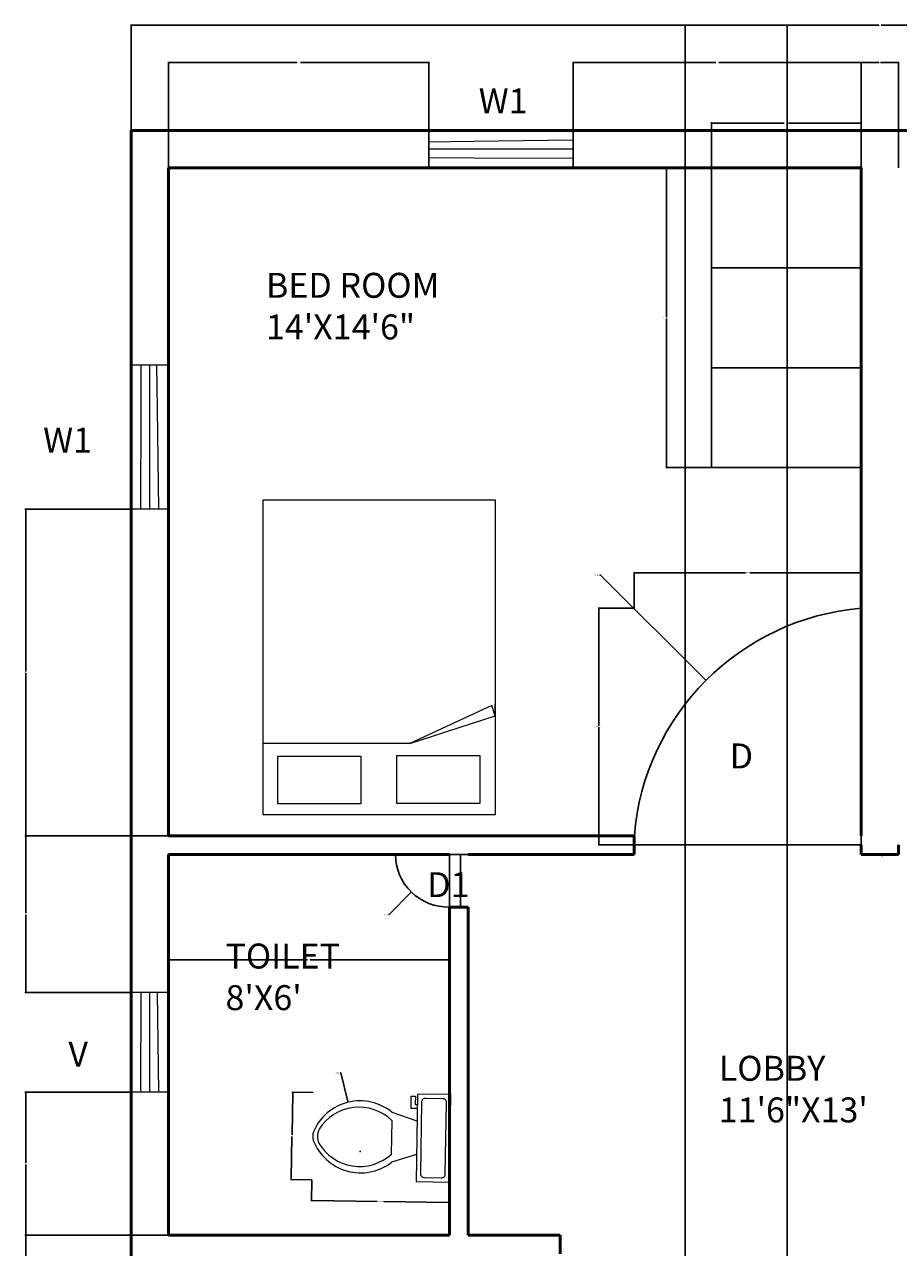
# Model space of a CAD drawing. Units: inches. Extents: x 2521 to 2933, y 1745 to 2276.
# Tile 3 of 4: x 2521 to 2731, y 1982 to 2276. Entities that reach past the tile are written whole.
import ezdxf

# ---------------------------------------------------------------- set-up
doc = ezdxf.new("R2010")
doc.units = ezdxf.units.IN
for name, color, linetype, lineweight in [('A-ANNO-DIMS', 2, 'Continuous', 18), ('A-ANNO-TEXT', 3, 'Continuous', 18), ('A-AREA-IDEN', 7, 'Continuous', 25), ('A-DOOR', 3, 'Continuous', 25), ('A-FLOR-CASE', 32, 'Continuous', 25), ('A-FLOR-FIXT', 9, 'Continuous', 18), ('A-FURN', 8, 'Continuous', 18), ('A-GLAZ', 4, 'Continuous', 20), ('A-WALL', 7, 'Continuous', 50)]:
    doc.layers.add(name, color=color, linetype=linetype, lineweight=lineweight)
doc.styles.get("Standard").update_dxf_attribs({"font": 'arial.ttf'})
doc.dimstyles.get("Standard").update_dxf_attribs({"dimtxt": 0.18, "dimasz": 0.18, "dimexe": 0.18, "dimexo": 0.0625, "dimgap": 0.09, "dimtad": 0, "dimtih": 1, "dimtoh": 1, "dimdec": 4, "dimzin": 0, "dimdsep": 46, "dimtxsty": 'Standard', "dimcen": 0.09, "dimadec": 0, "dimazin": 0, "dimtfac": 1, "dimtdec": 4, "dimtofl": 0, "dimtmove": 0, "dimatfit": 3, "dimfxl": 1, "dimtolj": 1, "dimtzin": 0, "dimarcsym": 0})

# ---------------------------------------------------------------- blocks, each defined once
blk = doc.blocks.new('Toilet - top')
for p, q in [((9.5, -6), (9.5, -2)), ((-10, -8.5), (-8, -8.5)), ((-10, -9.5), (-10, -8.5)), ((-8, -8.5), (-8, -8)), ((-7, -8), (-7, -9.5)), ((-4, -8), (-6, -14)), ((4, -8), (6, -14)), ((-7, -9.5), (-10, -9.5)), ((4, -14), (-4, -14))]:
    blk.add_line(p, q)
blk.add_lwpolyline([(10.5, -8), (10.5, 0), (-10.5, 0), (-10.5, -8)], close=True)
for points in [[(-9.5, -2), (-9.5, -6)], [(8.5, -1), (-8.5, -1)], [(-8.5, -7), (8.5, -7)]]:
    blk.add_lwpolyline(points)
for centre, radius, start, end in [((-8.62, -1.88), 0.884, 81.8699, 188.1301), ((8.62, -1.88), 0.884, 351.8699, 98.1301), ((-8.62, -6.12), 0.884, 171.8699, 278.1301), ((8.62, -6.12), 0.884, 261.8699, 8.1301), ((3.52, -21.58), 12.17, 141.4691, 247.9714), ((4.2, -21.82), 11.33, 136.3677, 238.9468), ((-3.52, -21.58), 12.17, 292.0284, 38.5307), ((-4.2, -21.82), 11.33, 301.053, 43.6321), ((0, -27.88), 4, 245.7318, 294.2682), ((0, -29), 4, 254.8605, 285.1395)]:
    blk.add_arc(centre, radius, start, end)
blk = doc.blocks.new('WINDOW-W1-LONG')
for p, q in [((0, 24), (0, 34.69)), ((0, 34.69), (9, 34.69)), ((2.4, 24), (2.44, 34.69)), ((4.5, 24), (4.5, 34.69)), ((6.37, 24), (6.23, 34.69)), ((9, 34.69), (9, 24)), ((0, 24), (0, 0)), ((2.32, 0), (2.4, 24)), ((4.5, 0), (4.5, 24)), ((6.68, 0), (6.37, 24)), ((9, 24), (9, 0)), ((9, 0), (0, 0))]:
    blk.add_line(p, q)
blk = doc.blocks.new('WINDOW-24')
for p, q in [((9, 24), (0, 24)), ((0, 24), (0, 0)), ((2.32, 0), (2.4, 24)), ((4.5, 0), (4.5, 24)), ((6.68, 0), (6.37, 24)), ((9, 24), (9, 0)), ((9, 0), (0, 0))]:
    blk.add_line(p, q)
blk = doc.blocks.new('DOOR-SINGLE-SWING')
for p, q in [((54.54, 0), (54.54, 56.86)), ((0, 0), (54.54, 0))]:
    blk.add_line(p, q)
blk.add_arc((59.46, -2.59), 59.65, 94.7338, 175.398)
blk = doc.blocks.new('BED-DOUBLE')
for p, q in [((55.72, 23.76), (55.72, 26.62)), ((54.9, 26.24), (35.19, 17.12)), ((35.19, 17.12), (55.72, 23.76)), ((55.72, 23.76), (54.9, 26.24)), ((35.19, 17.12), (0, 17.12))]:
    blk.add_line(p, q)
for points in [[(0, 75.73), (55.72, 75.73), (55.72, 0), (0, 0)], [(3.53, 14.11), (23.44, 14.11), (23.44, 2.6), (3.53, 2.6)], [(32.11, 14.25), (52.02, 14.25), (52.02, 2.74), (32.11, 2.74)]]:
    blk.add_lwpolyline(points, close=True)
blk = doc.blocks.new('CABINET-3-BAY')
for p, q in [((0, 0), (0, 72)), ((0, 48), (36, 48)), ((0, 24), (36, 24)), ((0, 0), (36, 0))]:
    blk.add_line(p, q)
blk = doc.blocks.new('*D15')
at = {"layer": 'A-ANNO-DIMS', "color": 0, "lineweight": -2, "transparency": 16777216}
for p, q in [((2686.45, 2241.28), (2675.53, 2241.28)), ((2675.71, 2241.1), (2675.71, 2205.46)), ((2675.71, 2169.46), (2675.71, 2205.1)), ((2686.45, 2169.28), (2675.53, 2169.28))]:
    blk.add_line(p, q, dxfattribs=at)
at = {"layer": 'A-ANNO-DIMS', "color": 0, "transparency": 16777216}
for points in [[(2675.68, 2241.1), (2675.74, 2241.1), (2675.71, 2241.28)], [(2675.68, 2169.46), (2675.74, 2169.46), (2675.71, 2169.28)]]:
    blk.add_solid(points, dxfattribs=at)
at = {"layer": 'Defpoints', "color": 0, "transparency": 16777216}
for p in [(2675.71, 2241.28), (2686.51, 2241.28), (2686.51, 2169.28)]:
    blk.add_point(p, dxfattribs=at)
at = {"layer": 'A-ANNO-DIMS', "color": 0, "transparency": 16777216, "insert": (2675.71, 2205.28), "char_height": 0.18, "attachment_point": 5}
blk.add_mtext('\\A1;CABINET 72 TYP.', dxfattribs=at)
blk = doc.blocks.new('*D16')
at = {"layer": 'A-ANNO-DIMS', "color": 0, "lineweight": -2, "transparency": 16777216}
for p, q in [((2686.51, 2241.34), (2686.51, 2252.26)), ((2686.69, 2252.08), (2703.98, 2252.08)), ((2722.33, 2252.08), (2705.04, 2252.08)), ((2722.51, 2241.34), (2722.51, 2252.26))]:
    blk.add_line(p, q, dxfattribs=at)
at = {"layer": 'A-ANNO-DIMS', "color": 0, "transparency": 16777216}
for points in [[(2686.69, 2252.11), (2686.69, 2252.05), (2686.51, 2252.08)], [(2722.33, 2252.11), (2722.33, 2252.05), (2722.51, 2252.08)]]:
    blk.add_solid(points, dxfattribs=at)
at = {"layer": 'Defpoints', "color": 0, "transparency": 16777216}
for p in [(2722.51, 2252.08), (2686.51, 2241.28), (2722.51, 2241.28)]:
    blk.add_point(p, dxfattribs=at)
at = {"layer": 'A-ANNO-DIMS', "color": 0, "transparency": 16777216, "insert": (2704.51, 2252.08), "char_height": 0.18, "attachment_point": 5}
blk.add_mtext('\\A1;36 TYP.', dxfattribs=at)
blk = doc.blocks.new('*D17')
at = {"layer": 'A-ANNO-DIMS', "color": 0, "lineweight": -2, "transparency": 16777216}
for p, q in [((2667.91, 2135.44), (2659.26, 2135.44)), ((2659.44, 2135.26), (2659.44, 2107.2)), ((2659.44, 2078.77), (2659.44, 2106.83)), ((2667.91, 2078.59), (2659.26, 2078.59))]:
    blk.add_line(p, q, dxfattribs=at)
at = {"layer": 'A-ANNO-DIMS', "color": 0, "transparency": 16777216}
for points in [[(2659.41, 2135.26), (2659.47, 2135.26), (2659.44, 2135.44)], [(2659.41, 2078.77), (2659.47, 2078.77), (2659.44, 2078.59)]]:
    blk.add_solid(points, dxfattribs=at)
at = {"layer": 'Defpoints', "color": 0, "transparency": 16777216}
for p in [(2659.44, 2135.44), (2667.97, 2135.44), (2667.97, 2078.59)]:
    blk.add_point(p, dxfattribs=at)
at = {"layer": 'A-ANNO-DIMS', "color": 0, "transparency": 16777216, "insert": (2659.44, 2107.01), "char_height": 0.18, "attachment_point": 5}
blk.add_mtext('\\A1;DOOR 57 TYP.', dxfattribs=at)
blk = doc.blocks.new('*D18')
at = {"layer": 'A-ANNO-DIMS', "color": 0, "lineweight": -2, "transparency": 16777216}
for p, q in [((2667.97, 2135.51), (2667.97, 2144.15)), ((2668.15, 2143.97), (2694.71, 2143.97)), ((2722.33, 2143.97), (2695.77, 2143.97)), ((2722.51, 2135.51), (2722.51, 2144.15))]:
    blk.add_line(p, q, dxfattribs=at)
at = {"layer": 'A-ANNO-DIMS', "color": 0, "transparency": 16777216}
for points in [[(2668.15, 2144), (2668.15, 2143.94), (2667.97, 2143.97)], [(2722.33, 2144), (2722.33, 2143.94), (2722.51, 2143.97)]]:
    blk.add_solid(points, dxfattribs=at)
at = {"layer": 'Defpoints', "color": 0, "transparency": 16777216}
for p in [(2722.51, 2143.97), (2667.97, 2135.44), (2722.51, 2135.44)]:
    blk.add_point(p, dxfattribs=at)
at = {"layer": 'A-ANNO-DIMS', "color": 0, "transparency": 16777216, "insert": (2695.24, 2143.97), "char_height": 0.18, "attachment_point": 5}
blk.add_mtext('\\A1;55 TYP.', dxfattribs=at)
blk = doc.blocks.new('*D19')
at = {"layer": 'A-ANNO-DIMS', "color": 0, "lineweight": -2, "transparency": 16777216}
for p, q in [((2590.47, 1998.02), (2590.38, 1992.94)), ((2623.51, 1997.47), (2623.42, 1992.4)), ((2590.57, 1993.12), (2606.13, 1992.86)), ((2623.25, 1992.58), (2607.68, 1992.84))]:
    blk.add_line(p, q, dxfattribs=at)
at = {"layer": 'A-ANNO-DIMS', "color": 0, "transparency": 16777216}
for points in [[(2590.57, 1993.15), (2590.57, 1993.09), (2590.39, 1993.12)], [(2623.25, 1992.61), (2623.25, 1992.55), (2623.43, 1992.58)]]:
    blk.add_solid(points, dxfattribs=at)
at = {"layer": 'Defpoints', "color": 0, "transparency": 16777216}
for p in [(2590.47, 1998.08), (2623.51, 1997.53), (2623.43, 1992.58)]:
    blk.add_point(p, dxfattribs=at)
at = {"layer": 'A-ANNO-DIMS', "color": 0, "transparency": 16777216, "insert": (2606.91, 1992.85), "char_height": 0.18, "attachment_point": 5}
blk.add_mtext('\\A1;WC 33 TYP.', dxfattribs=at)
blk = doc.blocks.new('*D20')
at = {"layer": 'A-ANNO-DIMS', "color": 0, "lineweight": -2, "transparency": 16777216}
for p, q in [((2590.75, 2019.08), (2585.68, 2019.16)), ((2585.85, 2018.98), (2585.69, 2008.84)), ((2585.51, 1998.34), (2585.68, 2008.48)), ((2590.4, 1998.08), (2585.33, 1998.16))]:
    blk.add_line(p, q, dxfattribs=at)
at = {"layer": 'A-ANNO-DIMS', "color": 0, "transparency": 16777216}
for points in [[(2585.82, 2018.98), (2585.88, 2018.98), (2585.86, 2019.16)], [(2585.48, 1998.34), (2585.54, 1998.34), (2585.51, 1998.16)]]:
    blk.add_solid(points, dxfattribs=at)
at = {"layer": 'Defpoints', "color": 0, "transparency": 16777216}
for p in [(2590.81, 2019.08), (2585.51, 1998.16), (2590.47, 1998.08)]:
    blk.add_point(p, dxfattribs=at)
at = {"layer": 'A-ANNO-DIMS', "color": 0, "transparency": 16777216, "insert": (2585.68, 2008.66), "char_height": 0.18, "attachment_point": 5}
blk.add_mtext('\\A1;21 TYP.', dxfattribs=at)
blk = doc.blocks.new('*D23')
at = {"layer": 'A-ANNO-DIMS', "color": 0, "lineweight": -2, "transparency": 16777216}
for p, q in [((2547.01, 2250.34), (2547.01, 2275.78)), ((2547.19, 2275.6), (2726.72, 2275.6)), ((2906.83, 2275.6), (2727.3, 2275.6)), ((2907.01, 2250.34), (2907.01, 2275.78))]:
    blk.add_line(p, q, dxfattribs=at)
at = {"layer": 'A-ANNO-DIMS', "color": 0, "transparency": 16777216}
for points in [[(2547.19, 2275.63), (2547.19, 2275.57), (2547.01, 2275.6)], [(2906.83, 2275.63), (2906.83, 2275.57), (2907.01, 2275.6)]]:
    blk.add_solid(points, dxfattribs=at)
at = {"layer": 'Defpoints', "color": 0, "transparency": 16777216}
for p in [(2907.01, 2275.6), (2547.01, 2250.28), (2907.01, 2250.28)]:
    blk.add_point(p, dxfattribs=at)
at = {"layer": 'A-ANNO-DIMS', "color": 0, "transparency": 16777216, "insert": (2727.01, 2275.6), "char_height": 0.18, "attachment_point": 5}
blk.add_mtext('\\A1;360', dxfattribs=at)
blk = doc.blocks.new('*D25')
at = {"layer": 'A-ANNO-DIMS', "color": 0, "lineweight": -2, "transparency": 16777216}
for p, q in [((2556.01, 2241.34), (2556.01, 2266.78)), ((2618.6, 2241.34), (2618.6, 2266.78)), ((2556.19, 2266.6), (2586.91, 2266.6)), ((2618.42, 2266.6), (2587.7, 2266.6))]:
    blk.add_line(p, q, dxfattribs=at)
at = {"layer": 'A-ANNO-DIMS', "color": 0, "transparency": 16777216}
for points in [[(2556.19, 2266.63), (2556.19, 2266.57), (2556.01, 2266.6)], [(2618.42, 2266.63), (2618.42, 2266.57), (2618.6, 2266.6)]]:
    blk.add_solid(points, dxfattribs=at)
at = {"layer": 'Defpoints', "color": 0, "transparency": 16777216}
for p in [(2618.6, 2266.6), (2556.01, 2241.28), (2618.6, 2241.28)]:
    blk.add_point(p, dxfattribs=at)
at = {"layer": 'A-ANNO-DIMS', "color": 0, "transparency": 16777216, "insert": (2587.31, 2266.6), "char_height": 0.18, "attachment_point": 5}
blk.add_mtext('\\A1;62.59', dxfattribs=at)
blk = doc.blocks.new('*D26')
at = {"layer": 'A-ANNO-DIMS', "color": 0, "lineweight": -2, "transparency": 16777216}
for p, q in [((2653.3, 2241.34), (2653.3, 2266.78)), ((2722.51, 2241.34), (2722.51, 2266.78)), ((2653.48, 2266.6), (2687.53, 2266.6)), ((2722.33, 2266.6), (2688.28, 2266.6))]:
    blk.add_line(p, q, dxfattribs=at)
at = {"layer": 'A-ANNO-DIMS', "color": 0, "transparency": 16777216}
for points in [[(2653.48, 2266.63), (2653.48, 2266.57), (2653.3, 2266.6)], [(2722.33, 2266.63), (2722.33, 2266.57), (2722.51, 2266.6)]]:
    blk.add_solid(points, dxfattribs=at)
at = {"layer": 'Defpoints', "color": 0, "transparency": 16777216}
for p in [(2722.51, 2266.6), (2653.3, 2241.28), (2722.51, 2241.28)]:
    blk.add_point(p, dxfattribs=at)
at = {"layer": 'A-ANNO-DIMS', "color": 0, "transparency": 16777216, "insert": (2687.9, 2266.6), "char_height": 0.18, "attachment_point": 5}
blk.add_mtext('\\A1;69.21', dxfattribs=at)
blk = doc.blocks.new('*D27')
at = {"layer": 'A-ANNO-DIMS', "color": 0, "lineweight": -2, "transparency": 16777216}
for p, q in [((2722.51, 2241.34), (2722.51, 2266.78)), ((2731.51, 2241.34), (2731.51, 2266.78)), ((2722.69, 2266.6), (2726.86, 2266.6)), ((2731.33, 2266.6), (2727.16, 2266.6))]:
    blk.add_line(p, q, dxfattribs=at)
at = {"layer": 'A-ANNO-DIMS', "color": 0, "transparency": 16777216}
for points in [[(2722.69, 2266.63), (2722.69, 2266.57), (2722.51, 2266.6)], [(2731.33, 2266.63), (2731.33, 2266.57), (2731.51, 2266.6)]]:
    blk.add_solid(points, dxfattribs=at)
at = {"layer": 'Defpoints', "color": 0, "transparency": 16777216}
for p in [(2731.51, 2266.6), (2722.51, 2241.28), (2731.51, 2241.28)]:
    blk.add_point(p, dxfattribs=at)
at = {"layer": 'A-ANNO-DIMS', "color": 0, "transparency": 16777216, "insert": (2727.01, 2266.6), "char_height": 0.18, "attachment_point": 5}
blk.add_mtext('\\A1;9', dxfattribs=at)
blk = doc.blocks.new('*D31')
at = {"layer": 'A-ANNO-DIMS', "color": 0, "lineweight": -2, "transparency": 16777216}
for p, q in [((2555.95, 1984.78), (2521.51, 1984.78)), ((2521.69, 1984.6), (2521.69, 1937.71)), ((2521.69, 1890.46), (2521.69, 1937.35)), ((2555.95, 1890.28), (2521.51, 1890.28))]:
    blk.add_line(p, q, dxfattribs=at)
at = {"layer": 'A-ANNO-DIMS', "color": 0, "transparency": 16777216}
for points in [[(2521.66, 1984.6), (2521.72, 1984.6), (2521.69, 1984.78)], [(2521.66, 1890.46), (2521.72, 1890.46), (2521.69, 1890.28)]]:
    blk.add_solid(points, dxfattribs=at)
at = {"layer": 'Defpoints', "color": 0, "transparency": 16777216}
for p in [(2521.69, 1984.78), (2556.01, 1984.78), (2556.01, 1890.28)]:
    blk.add_point(p, dxfattribs=at)
at = {"layer": 'A-ANNO-DIMS', "color": 0, "transparency": 16777216, "insert": (2521.69, 1937.53), "char_height": 0.18, "attachment_point": 5}
blk.add_mtext('\\A1;94.5', dxfattribs=at)
blk = doc.blocks.new('*D32')
at = {"layer": 'A-ANNO-DIMS', "color": 0, "lineweight": -2, "transparency": 16777216}
for p, q in [((2546.95, 2019.1), (2521.51, 2019.1)), ((2521.69, 2018.92), (2521.69, 2002.12)), ((2521.69, 1984.96), (2521.69, 2001.76)), ((2555.95, 1984.78), (2521.51, 1984.78))]:
    blk.add_line(p, q, dxfattribs=at)
at = {"layer": 'A-ANNO-DIMS', "color": 0, "transparency": 16777216}
for points in [[(2521.66, 2018.92), (2521.72, 2018.92), (2521.69, 2019.1)], [(2521.66, 1984.96), (2521.72, 1984.96), (2521.69, 1984.78)]]:
    blk.add_solid(points, dxfattribs=at)
at = {"layer": 'Defpoints', "color": 0, "transparency": 16777216}
for p in [(2521.69, 2019.1), (2547.01, 2019.1), (2556.01, 1984.78)]:
    blk.add_point(p, dxfattribs=at)
at = {"layer": 'A-ANNO-DIMS', "color": 0, "transparency": 16777216, "insert": (2521.69, 2001.94), "char_height": 0.18, "attachment_point": 5}
blk.add_mtext('\\A1;34.32', dxfattribs=at)
blk = doc.blocks.new('*D33')
at = {"layer": 'A-ANNO-DIMS', "color": 0, "lineweight": -2, "transparency": 16777216}
for p, q in [((2555.95, 2080.78), (2521.51, 2080.78)), ((2521.69, 2080.6), (2521.69, 2062.12)), ((2521.69, 2043.28), (2521.69, 2061.76)), ((2546.95, 2043.1), (2521.51, 2043.1))]:
    blk.add_line(p, q, dxfattribs=at)
at = {"layer": 'A-ANNO-DIMS', "color": 0, "transparency": 16777216}
for points in [[(2521.66, 2080.6), (2521.72, 2080.6), (2521.69, 2080.78)], [(2521.66, 2043.28), (2521.72, 2043.28), (2521.69, 2043.1)]]:
    blk.add_solid(points, dxfattribs=at)
at = {"layer": 'Defpoints', "color": 0, "transparency": 16777216}
for p in [(2521.69, 2080.78), (2556.01, 2080.78), (2547.01, 2043.1)]:
    blk.add_point(p, dxfattribs=at)
at = {"layer": 'A-ANNO-DIMS', "color": 0, "transparency": 16777216, "insert": (2521.69, 2061.94), "char_height": 0.18, "attachment_point": 5}
blk.add_mtext('\\A1;37.68', dxfattribs=at)
blk = doc.blocks.new('*D34')
at = {"layer": 'A-ANNO-DIMS', "color": 0, "lineweight": -2, "transparency": 16777216}
for p, q in [((2546.95, 2159.3), (2521.51, 2159.3)), ((2521.69, 2159.12), (2521.69, 2120.22)), ((2521.69, 2080.96), (2521.69, 2119.86)), ((2555.95, 2080.78), (2521.51, 2080.78))]:
    blk.add_line(p, q, dxfattribs=at)
at = {"layer": 'A-ANNO-DIMS', "color": 0, "transparency": 16777216}
for points in [[(2521.66, 2159.12), (2521.72, 2159.12), (2521.69, 2159.3)], [(2521.66, 2080.96), (2521.72, 2080.96), (2521.69, 2080.78)]]:
    blk.add_solid(points, dxfattribs=at)
at = {"layer": 'Defpoints', "color": 0, "transparency": 16777216}
for p in [(2521.69, 2159.3), (2547.01, 2159.3), (2556.01, 2080.78)]:
    blk.add_point(p, dxfattribs=at)
at = {"layer": 'A-ANNO-DIMS', "color": 0, "transparency": 16777216, "insert": (2521.69, 2120.04), "char_height": 0.18, "attachment_point": 5}
blk.add_mtext('\\A1;78.51', dxfattribs=at)
blk = doc.blocks.new('*D48')
at = {"layer": 'A-ANNO-DIMS', "color": 0, "lineweight": -2, "transparency": 16777216}
for p, q in [((2556.01, 2076.22), (2556.01, 2050.78)), ((2623.51, 2076.22), (2623.51, 2050.78)), ((2556.19, 2050.96), (2589.43, 2050.96)), ((2623.33, 2050.96), (2590.08, 2050.96))]:
    blk.add_line(p, q, dxfattribs=at)
at = {"layer": 'A-ANNO-DIMS', "color": 0, "transparency": 16777216}
for points in [[(2556.19, 2050.99), (2556.19, 2050.93), (2556.01, 2050.96)], [(2623.33, 2050.99), (2623.33, 2050.93), (2623.51, 2050.96)]]:
    blk.add_solid(points, dxfattribs=at)
at = {"layer": 'Defpoints', "color": 0, "transparency": 16777216}
for p in [(2556.01, 2076.28), (2623.51, 2076.28), (2556.01, 2050.96)]:
    blk.add_point(p, dxfattribs=at)
at = {"layer": 'A-ANNO-DIMS', "color": 0, "transparency": 16777216, "insert": (2589.76, 2050.96), "char_height": 0.18, "attachment_point": 5}
blk.add_mtext('\\A1;67.5', dxfattribs=at)
blk = doc.blocks.new('*D55')
at = {"layer": 'A-ANNO-DIMS', "color": 0, "lineweight": -2, "transparency": 16777216}
for p, q in [((2680.23, 1804.66), (2680.23, 2275.78)), ((2680.41, 2275.6), (2692.15, 2275.6)), ((2704.55, 2275.6), (2692.81, 2275.6)), ((2704.73, 1859.95), (2704.73, 2275.78))]:
    blk.add_line(p, q, dxfattribs=at)
at = {"layer": 'A-ANNO-DIMS', "color": 0, "transparency": 16777216}
for points in [[(2680.41, 2275.63), (2680.41, 2275.57), (2680.23, 2275.6)], [(2704.55, 2275.63), (2704.55, 2275.57), (2704.73, 2275.6)]]:
    blk.add_solid(points, dxfattribs=at)
at = {"layer": 'Defpoints', "color": 0, "transparency": 16777216}
for p in [(2704.73, 2275.6), (2704.73, 1859.89), (2680.23, 1804.6)]:
    blk.add_point(p, dxfattribs=at)
at = {"layer": 'A-ANNO-DIMS', "color": 0, "transparency": 16777216, "insert": (2692.48, 2275.6), "char_height": 0.18, "attachment_point": 5}
blk.add_mtext('\\A1;24.5', dxfattribs=at)
blk = doc.blocks.new('*D61')
at = {"layer": 'A-ANNO-DIMS', "color": 0, "lineweight": -2, "transparency": 16777216}
for p, q in [((2659.69, 2143.41), (2659.87, 2143.41)), ((2659.87, 2143.41), (2685.08, 2118.25)), ((2727.34, 2076), (2727.52, 2076)), ((2727.43, 2075.91), (2727.43, 2076.09))]:
    blk.add_line(p, q, dxfattribs=at)
at = {"layer": 'A-ANNO-DIMS', "color": 0, "transparency": 16777216}
blk.add_solid([(2685.1, 2118.28), (2685.06, 2118.23), (2685.2, 2118.13)], dxfattribs=at)
at = {"layer": 'Defpoints', "color": 0, "transparency": 16777216}
for p in [(2685.2, 2118.13), (2727.43, 2076)]:
    blk.add_point(p, dxfattribs=at)
at = {"layer": 'A-ANNO-DIMS', "color": 0, "transparency": 16777216, "insert": (2659.01, 2143.41), "char_height": 0.18, "attachment_point": 5}
blk.add_mtext('\\A1;2X R59.65', dxfattribs=at)
blk = doc.blocks.new('*D63')
at = {"layer": 'A-ANNO-DIMS', "color": 0, "lineweight": -2, "transparency": 16777216}
for p, q in [((2623.12, 2076.24), (2623.3, 2076.24)), ((2623.21, 2076.15), (2623.21, 2076.33)), ((2609.07, 2061.81), (2614.25, 2067.1)), ((2608.89, 2061.81), (2609.07, 2061.81))]:
    blk.add_line(p, q, dxfattribs=at)
at = {"layer": 'A-ANNO-DIMS', "color": 0, "transparency": 16777216}
blk.add_solid([(2614.23, 2067.12), (2614.27, 2067.07), (2614.38, 2067.22)], dxfattribs=at)
at = {"layer": 'Defpoints', "color": 0, "transparency": 16777216}
for p in [(2623.21, 2076.24), (2614.38, 2067.22)]:
    blk.add_point(p, dxfattribs=at)
at = {"layer": 'A-ANNO-DIMS', "color": 0, "transparency": 16777216, "insert": (2608.34, 2061.81), "char_height": 0.18, "attachment_point": 5}
blk.add_mtext('\\A1;R12.627', dxfattribs=at)
blk = doc.blocks.new('*D64')
at = {"layer": 'A-ANNO-DIMS', "color": 0, "lineweight": -2, "transparency": 16777216}
for p, q in [((2597.23, 2023.78), (2597.41, 2023.78)), ((2597.41, 2023.78), (2599.11, 2016.86)), ((2601.96, 2004.87), (2602.14, 2004.87)), ((2602.05, 2004.78), (2602.05, 2004.96))]:
    blk.add_line(p, q, dxfattribs=at)
at = {"layer": 'A-ANNO-DIMS', "color": 0, "transparency": 16777216}
blk.add_solid([(2599.13, 2016.87), (2599.08, 2016.86), (2599.15, 2016.69)], dxfattribs=at)
at = {"layer": 'Defpoints', "color": 0, "transparency": 16777216}
for p in [(2599.15, 2016.69), (2602.05, 2004.87)]:
    blk.add_point(p, dxfattribs=at)
at = {"layer": 'A-ANNO-DIMS', "color": 0, "transparency": 16777216, "insert": (2596.55, 2023.78), "char_height": 0.18, "attachment_point": 5}
blk.add_mtext('\\A1;4X R12.17', dxfattribs=at)

msp = doc.modelspace()

# ---------------------------------------------------------------- linework, layer by layer
at = {"layer": 'A-DOOR'}
for p, q in [((2610.5844, 2076.2819), (2626.1881, 2076.2819)), ((2626.1881, 2076.2819), (2626.1881, 2063.9735)), ((2628.009, 2076.2819), (2626.1881, 2076.2819)), ((2626.1881, 2063.9735), (2626.1881, 2063.6098))]:
    msp.add_line(p, q, dxfattribs=at)
msp.add_arc((2623.2111, 2076.2443), 12.6267, 179.82927, 271.352003, dxfattribs=at)
at = {"layer": 'A-WALL'}
for p, q in [((2547.009, 2250.2819), (2907.009, 2250.2819)), ((2547.009, 1770.2819), (2547.009, 2250.2819)), ((2556.009, 2241.2819), (2722.509, 2241.2819)), ((2556.009, 2080.7819), (2556.009, 2241.2819)), ((2722.509, 2080.7819), (2722.509, 2241.2819)), ((2667.9735, 2080.7819), (2556.009, 2080.7819)), ((2667.9735, 2080.7819), (2667.9735, 2076.2819)), ((2722.509, 2078.585), (2722.509, 2076.2819)), ((2731.479, 2078.585), (2731.479, 2076.2819)), ((2556.009, 2076.2819), (2556.009, 1984.7819)), ((2556.009, 1984.7819), (2556.009, 2076.2819)), ((2623.509, 2076.2819), (2556.009, 2076.2819)), ((2667.9735, 2076.2819), (2628.009, 2076.2819)), ((2722.509, 2076.2819), (2731.479, 2076.2819)), ((2623.509, 1984.7819), (2623.509, 2063.621)), ((2623.509, 2063.621), (2628.009, 2063.6022)), ((2628.009, 1984.7819), (2628.009, 2063.6022)), ((2556.009, 1984.7819), (2623.509, 1984.7819)), ((2628.009, 1984.7819), (2650.1821, 1984.7819)), ((2650.1821, 1980.2819), (2650.1821, 1984.7819))]:
    msp.add_line(p, q, dxfattribs=at)

# ---------------------------------------------------------------- block references
at = {"layer": 'A-DOOR'}
msp.add_blockref('DOOR-SINGLE-SWING', (2667.973, 2078.585), dxfattribs=at)
at = {"layer": 'A-FLOR-CASE'}
msp.add_blockref('CABINET-3-BAY', (2686.509, 2169.282), dxfattribs=at)
at = {"layer": 'A-FLOR-FIXT', "rotation": 269.0579063208954}
msp.add_blockref('Toilet - top', (2623.6817, 2008.0334), dxfattribs=at)
at = {"layer": 'A-FURN'}
msp.add_blockref('BED-DOUBLE', (2578.788, 2085.81), dxfattribs=at)
at = {"layer": 'A-GLAZ', "rotation": 89.99999999999793}
msp.add_blockref('WINDOW-W1-LONG', (2653.2972, 2241.2819), dxfattribs=at)
at = {"layer": 'A-GLAZ'}
for name, p in [('WINDOW-W1-LONG', (2547.009, 2159.295)), ('WINDOW-24', (2547.009, 2019.1009))]:
    msp.add_blockref(name, p, dxfattribs=at)

# ---------------------------------------------------------------- texts
at = {"layer": 'A-ANNO-TEXT', "char_height": 6, "attachment_point": 1}
for s, width, insert in [('W1', 10.7254, (2630.5716, 2260.4013)), ('W1', 15.32248, (2525.8777, 2178.8496)), ('D', 9.612648, (2690.8877, 2102.9455)), ('D1', 3.641626, (2618.1873, 2072.0082)), ('V', 9.677367, (2531.9417, 2031.2929))]:
    msp.add_mtext_dynamic_manual_height_columns(s, width=width, gutter_width=5.8967, heights=[0], dxfattribs=dict(at, insert=insert))
at = {"layer": 'A-AREA-IDEN', "char_height": 6, "attachment_point": 1}
for s, width, insert in [('BED ROOM \\P14\'X14\'6"', 71.736558, (2579.4344, 2216.0769)), ("TOILET\\P8'X6'", 29.917519, (2569.7047, 2054.8508)), ('LOBBY\\P11\'6"X13\'', 59.103054, (2688.2675, 2027.8638))]:
    msp.add_mtext_dynamic_manual_height_columns(s, width=width, gutter_width=5.8967, heights=[0], dxfattribs=dict(at, insert=insert))

# ---------------------------------------------------------------- dimensions: what is measured, and where the dimension line sits
at = {"layer": 'A-ANNO-DIMS'}
for base, p1, p2, override, picture, middle in [((2907.009, 2275.6019), (2547.009, 2250.2819), (2907.009, 2250.2819), {"dimdec": 0, "dimlfac": 1, "dimrnd": 0, "dimzin": 0, "dimdsep": 46, "dimlunit": 2}, '*D23', (2727.009, 2275.6019)), ((2704.7306, 2275.6019), (2680.2296, 1804.5971), (2704.7306, 1859.892), {"dimdec": 1, "dimlfac": 1, "dimrnd": 0, "dimzin": 0, "dimdsep": 46, "dimlunit": 2}, '*D55', (2692.4801, 2275.6019)), ((2722.509, 2266.6019), (2653.297, 2241.2819), (2722.509, 2241.2819), {"dimdec": 2, "dimlfac": 1, "dimrnd": 0, "dimzin": 0, "dimdsep": 46, "dimlunit": 2}, '*D26', (2687.903, 2266.6019)), ((2731.509, 2266.6019), (2722.509, 2241.2819), (2731.509, 2241.2819), {"dimdec": 0, "dimlfac": 1, "dimrnd": 0, "dimzin": 0, "dimdsep": 46, "dimlunit": 2}, '*D27', (2727.009, 2266.6019))]:
    dim = msp.add_linear_dim(base=base, p1=p1, p2=p2, dimstyle='Standard', override=override, dxfattribs=at)
    dim.commit()
    dim.dimension.update_dxf_attribs({"geometry": picture, "text_midpoint": middle})
for base, p1, p2, angle, override, picture, middle in [((2618.6027, 2266.6019), (2556.009, 2241.2819), (2618.6027, 2241.2819), 0, {"dimdec": 2, "dimlfac": 1, "dimrnd": 0, "dimzin": 0, "dimdsep": 46, "dimlunit": 2}, '*D25', (2587.3059, 2266.6019)), ((2521.689, 2159.2952), (2556.009, 2080.7819), (2547.009, 2159.2952), 90, {"dimdec": 2, "dimlfac": 1, "dimrnd": 0, "dimzin": 0, "dimdsep": 46, "dimlunit": 2}, '*D34', (2521.689, 2120.0386)), ((2521.689, 2080.7819), (2547.009, 2043.1006), (2556.009, 2080.7819), 90, {"dimdec": 2, "dimlfac": 1, "dimrnd": 0, "dimzin": 0, "dimdsep": 46, "dimlunit": 2}, '*D33', (2521.689, 2061.9413)), ((2556.009, 2050.9619), (2623.509, 2076.2819), (2556.009, 2076.2819), 180, {"dimdec": 1, "dimlfac": 1, "dimrnd": 0, "dimzin": 0, "dimdsep": 46, "dimlunit": 2}, '*D48', (2589.759, 2050.9619)), ((2521.689, 2019.1006), (2556.009, 1984.7819), (2547.009, 2019.1006), 90, {"dimdec": 2, "dimlfac": 1, "dimrnd": 0, "dimzin": 0, "dimdsep": 46, "dimlunit": 2}, '*D32', (2521.689, 2001.9413)), ((2521.689, 1984.7819), (2556.009, 1890.2819), (2556.009, 1984.7819), 90, {"dimdec": 1, "dimlfac": 1, "dimrnd": 0, "dimzin": 0, "dimdsep": 46, "dimlunit": 2}, '*D31', (2521.689, 1937.5319))]:
    dim = msp.add_linear_dim(base=base, p1=p1, p2=p2, angle=angle, dimstyle='Standard', override=override, dxfattribs=at)
    dim.commit()
    dim.dimension.update_dxf_attribs({"geometry": picture, "text_midpoint": middle})
for base, p1, p2, picture, middle in [((2722.509, 2252.0819), (2686.509, 2241.2819), (2722.509, 2241.2819), '*D16', (2704.509, 2252.0819)), ((2722.509, 2143.9717), (2667.9735, 2135.443), (2722.509, 2135.443), '*D18', (2695.2413, 2143.9717))]:
    dim = msp.add_linear_dim(base=base, p1=p1, p2=p2, text='<> TYP.', dimstyle='Standard', override={"dimdec": 0, "dimlfac": 1, "dimrnd": 0, "dimzin": 0, "dimdsep": 46, "dimlunit": 2}, dxfattribs=at)
    dim.commit()
    dim.dimension.update_dxf_attribs({"geometry": picture, "text_midpoint": middle})
for base, p1, p2, angle, text, picture, middle in [((2675.709, 2241.2819), (2686.509, 2169.2819), (2686.509, 2241.2819), 90, 'CABINET <> TYP.', '*D15', (2675.709, 2205.2819)), ((2659.4448, 2135.443), (2667.9735, 2078.585), (2667.9735, 2135.443), 90, 'DOOR <> TYP.', '*D17', (2659.4448, 2107.014)), ((2585.511, 1998.1597), (2590.8125, 2019.0754), (2590.4673, 1998.0782), 269.057906, '<> TYP.', '*D20', (2585.6836, 2008.6583)), ((2623.4275, 1992.5786), (2590.4673, 1998.0782), (2623.509, 1997.5349), 359.057906, 'WC <> TYP.', '*D19', (2606.9066, 1992.8503))]:
    dim = msp.add_linear_dim(base=base, p1=p1, p2=p2, angle=angle, text=text, dimstyle='Standard', override={"dimdec": 0, "dimlfac": 1, "dimrnd": 0, "dimzin": 0, "dimdsep": 46, "dimlunit": 2}, dxfattribs=at)
    dim.commit()
    dim.dimension.update_dxf_attribs({"geometry": picture, "text_midpoint": middle})
for center, mpoint, text, picture, middle in [((2727.4318, 2075.9959), (2685.2041, 2118.1269), '2X <>', '*D61', (2659.0122, 2143.4055)), ((2602.0462, 2004.8692), (2599.148, 2016.688), '4X <>', '*D64', (2596.5522, 2023.7793))]:
    dim = msp.add_radius_dim(center=center, mpoint=mpoint, text=text, dimstyle='Standard', override={"dimdec": 2, "dimlfac": 1, "dimrnd": 0, "dimzin": 0, "dimdsep": 46, "dimlunit": 2}, dxfattribs=at)
    dim.commit()
    dim.dimension.update_dxf_attribs({"geometry": picture, "text_midpoint": middle, "dimtype": 164})
dim = msp.add_radius_dim(center=(2623.2111, 2076.2443), mpoint=(2614.3752, 2067.2242), dimstyle='Standard', override={"dimdec": 3, "dimlfac": 1, "dimrnd": 0, "dimzin": 0, "dimdsep": 46, "dimlunit": 2}, dxfattribs=at)
dim.commit()
dim.dimension.update_dxf_attribs({"geometry": '*D63', "text_midpoint": (2608.3439, 2061.8122), "dimtype": 164})

doc.saveas('drawing.dxf')
